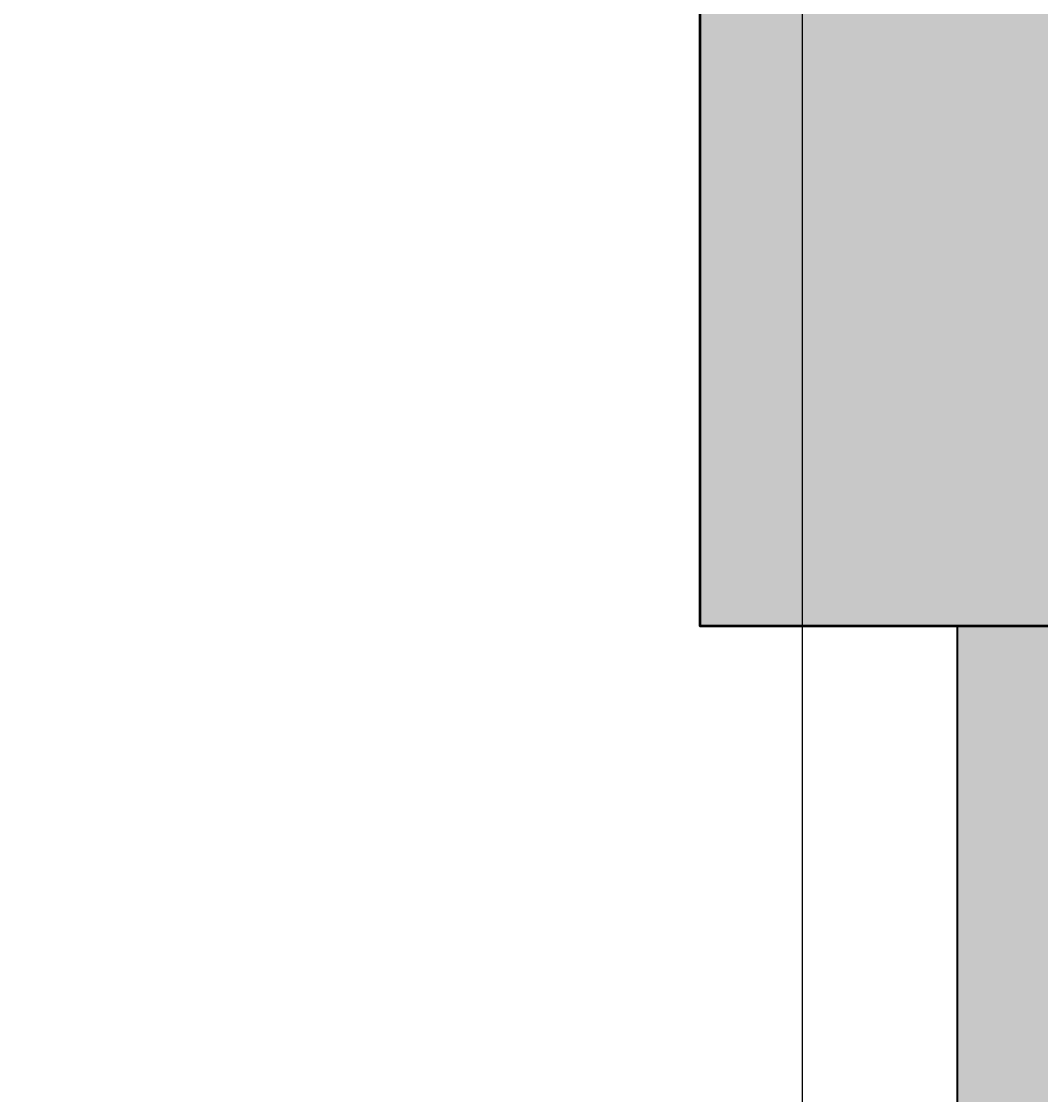
# Model space of a CAD drawing. Units: inches. Extents: x 1998 to 2588, y 1139 to 1977.
# Tile 28 of 134: x 2316 to 2344, y 1456 to 1484. Entities that reach past the tile are written whole.
import ezdxf

# ---------------------------------------------------------------- set-up
doc = ezdxf.new("R2010")
doc.units = ezdxf.units.IN
for name, color, linetype, lineweight in [('A-ANNO-DIMS', 2, 'Continuous', 18), ('A-COLS-PATT', 250, 'Continuous', 13), ('A-WALL-PATT', 252, 'Continuous', 13), ('COLUMN', 10, 'Continuous', 50), ('WALL', 200, 'Continuous', 35)]:
    doc.layers.add(name, color=color, linetype=linetype, lineweight=lineweight)
doc.styles.get("Standard").update_dxf_attribs({"font": 'arial.ttf'})
doc.dimstyles.get("Standard").update_dxf_attribs({"dimtxt": 0.18, "dimasz": 0.18, "dimexe": 0.18, "dimexo": 0.0625, "dimgap": 0.09, "dimtad": 0, "dimtih": 1, "dimtoh": 1, "dimdec": 4, "dimzin": 0, "dimdsep": 46, "dimtxsty": 'Standard', "dimcen": 0.09, "dimadec": 0, "dimazin": 0, "dimtfac": 1, "dimtdec": 4, "dimtofl": 0, "dimtmove": 0, "dimatfit": 3, "dimfxl": 1, "dimtolj": 1, "dimtzin": 0, "dimarcsym": 0})

# ---------------------------------------------------------------- blocks, each defined once
blk = doc.blocks.new('*D23')
at = {"layer": 'A-ANNO-DIMS', "color": 0, "lineweight": -2, "transparency": 16777216}
for p, q in [((2549.179, 1476.17), (2549.179, 1138.602)), ((2059.473, 1413.17), (2059.473, 1138.602)), ((2059.653, 1138.782), (2303.928, 1138.782)), ((2548.999, 1138.782), (2304.723, 1138.782))]:
    blk.add_line(p, q, dxfattribs=at)
at = {"layer": 'A-ANNO-DIMS', "color": 0, "transparency": 16777216}
for points in [[(2059.653, 1138.812), (2059.653, 1138.752), (2059.473, 1138.782)], [(2548.999, 1138.812), (2548.999, 1138.752), (2549.179, 1138.782)]]:
    blk.add_solid(points, dxfattribs=at)
at = {"layer": 'Defpoints', "color": 0, "transparency": 16777216}
for p in [(2549.179, 1476.232), (2059.473, 1413.232), (2549.179, 1138.782)]:
    blk.add_point(p, dxfattribs=at)
at = {"layer": 'A-ANNO-DIMS', "color": 0, "transparency": 16777216, "insert": (2304.326, 1138.782), "char_height": 0.18, "attachment_point": 5}
blk.add_mtext('\\A1;489.7', dxfattribs=at)
blk = doc.blocks.new('*D44')
at = {"layer": 'A-ANNO-DIMS', "color": 0, "lineweight": -2, "transparency": 16777216}
for p, q in [((2295.414, 1588.67), (2295.414, 1138.602)), ((2337.287, 1588.67), (2337.287, 1138.602)), ((2295.594, 1138.782), (2315.953, 1138.782)), ((2337.107, 1138.782), (2316.748, 1138.782))]:
    blk.add_line(p, q, dxfattribs=at)
at = {"layer": 'A-ANNO-DIMS', "color": 0, "transparency": 16777216}
for points in [[(2295.594, 1138.812), (2295.594, 1138.752), (2295.414, 1138.782)], [(2337.107, 1138.812), (2337.107, 1138.752), (2337.287, 1138.782)]]:
    blk.add_solid(points, dxfattribs=at)
at = {"layer": 'Defpoints', "color": 0, "transparency": 16777216}
for p in [(2295.414, 1588.732), (2337.287, 1588.732), (2337.287, 1138.782)]:
    blk.add_point(p, dxfattribs=at)
at = {"layer": 'A-ANNO-DIMS', "color": 0, "transparency": 16777216, "insert": (2316.35, 1138.782), "char_height": 0.18, "attachment_point": 5}
blk.add_mtext('\\A1;41.87', dxfattribs=at)

msp = doc.modelspace()

# ---------------------------------------------------------------- hatches: boundary and pattern name
at = {"layer": 'A-COLS-PATT'}
h = msp.add_hatch(color=256, dxfattribs=at)
h.dxf.hatch_style = 1
h.paths.add_polyline_path([(2099.4125, 1888.7324), (2087.9729, 1888.7324), (2087.9729, 1868.3278), (2099.4125, 1868.3278)])
h.paths.add_polyline_path([(2234.4125, 1888.7324), (2222.9729, 1888.7324), (2222.9729, 1868.3278), (2234.4125, 1868.3278)])
h.paths.add_polyline_path([(2341.4729, 1886.637), (2330.0332, 1886.637), (2330.0332, 1866.2324), (2341.4729, 1866.2324)])
h.paths.add_polyline_path([(2507.8006, 1882.7324), (2487.396, 1882.7324), (2487.396, 1871.2927), (2507.8006, 1871.2927)])
h.paths.add_polyline_path([(2510.9729, 1766.672), (2490.5682, 1766.672), (2490.5682, 1755.2324), (2510.9729, 1755.2324)])
h.paths.add_polyline_path([(2345.9729, 1759.7324), (2334.5332, 1759.7324), (2334.5332, 1739.3278), (2345.9729, 1739.3278)])
h.paths.add_polyline_path([(2234.4125, 1774.3318), (2222.9729, 1774.3318), (2222.9729, 1753.9272), (2234.4125, 1753.9272)])
h.paths.add_polyline_path([(2099.4125, 1775.637), (2087.9729, 1775.637), (2087.9729, 1755.2324), (2099.4125, 1755.2324)])
h.paths.add_polyline_path([(2098.0956, 1593.7241), (2077.691, 1593.7241), (2077.691, 1582.2845), (2098.0956, 1582.2845)])
h.paths.add_polyline_path([(2227.4729, 1604.637), (2216.0332, 1604.637), (2216.0332, 1584.2324), (2227.4729, 1584.2324)])
h.paths.add_polyline_path([(2345.9729, 1647.5211), (2334.5332, 1647.5211), (2334.5332, 1627.1165), (2345.9729, 1627.1165)])
h.paths.add_polyline_path([(2522.3775, 1641.2324), (2501.9729, 1641.2324), (2501.9729, 1629.7927), (2522.3775, 1629.7927)])
h.paths.add_polyline_path([(2522.3775, 1480.7324), (2501.9729, 1480.7324), (2501.9729, 1469.2927), (2522.3775, 1469.2927)])
h.paths.add_polyline_path([(2345.9729, 1488.5616), (2334.5332, 1488.5616), (2334.5332, 1468.1569), (2345.9729, 1468.1569)])
h.paths.add_polyline_path([(2234.4125, 1486.137), (2227.4729, 1486.137), (2227.4729, 1465.7324), (2234.4125, 1465.7324)])
h.paths.add_polyline_path([(2227.4729, 1486.137), (2222.9729, 1486.137), (2222.9729, 1465.7324), (2227.4729, 1465.7324)])
h.paths.add_polyline_path([(2108.3775, 1470.2324), (2087.9729, 1470.2324), (2087.9729, 1458.7927), (2108.3775, 1458.7927)])
h.paths.add_polyline_path([(2096.9729, 1365.5012), (2087.9729, 1365.5012), (2087.9729, 1345.0966), (2096.9729, 1345.0966)])
h.paths.add_polyline_path([(2087.9729, 1365.5012), (2085.5332, 1365.5012), (2085.5332, 1345.0966), (2087.9729, 1345.0966)])
h.paths.add_polyline_path([(2234.4125, 1285.137), (2222.9729, 1285.137), (2222.9729, 1264.7324), (2234.4125, 1264.7324)])
h.paths.add_polyline_path([(2345.9729, 1285.137), (2334.5332, 1285.137), (2334.5332, 1264.7324), (2345.9729, 1264.7324)])
h.paths.add_polyline_path([(2503.1458, 1240.172), (2482.7412, 1240.172), (2482.7412, 1228.7324), (2503.1458, 1228.7324)])
h.paths.add_polyline_path([(2510.9729, 1369.172), (2490.5682, 1369.172), (2490.5682, 1357.7324), (2510.9729, 1357.7324)])
at = {"layer": 'A-WALL-PATT'}
h = msp.add_hatch(color=256, dxfattribs=at)
h.dxf.hatch_style = 1
h.paths.add_polyline_path([(2222.9729, 1888.7324), (2099.4125, 1888.7324), (2099.4125, 1879.7324), (2222.9729, 1879.7324)])
h.paths.add_polyline_path([(2096.9729, 1868.3278), (2087.9729, 1868.3278), (2087.9729, 1775.637), (2096.9729, 1775.637)])
h.paths.add_polyline_path([(2227.4729, 1868.3278), (2222.9729, 1868.3278), (2222.9729, 1774.3318), (2227.4729, 1774.3318)])
h.paths.add_polyline_path([(2188.3019, 1759.7324), (2138.6074, 1759.7324), (2099.4125, 1759.7324), (2099.4125, 1755.2324), (2176.9729, 1755.2324), (2188.3019, 1755.2324)])
h.paths.add_polyline_path([(2087.9729, 1759.7324), (2059.4729, 1759.7324), (2059.4729, 1702.7324), (2087.9729, 1702.7324), (2087.9729, 1707.2324), (2063.9729, 1707.2324), (2063.9729, 1755.2324), (2087.9729, 1755.2324)])
h.paths.add_polyline_path([(2096.9729, 1755.2324), (2087.9729, 1755.2324), (2087.9729, 1707.2324), (2096.9729, 1707.2324)])
h.paths.add_polyline_path([(2187.0461, 1707.2324), (2105.9729, 1707.2324), (2096.9729, 1707.2324), (2087.9729, 1707.2324), (2087.9729, 1702.7324), (2105.9729, 1702.7324), (2114.9729, 1702.7324), (2187.0461, 1702.7324)])
h.paths.add_polyline_path([(2181.4729, 1719.2028), (2176.9729, 1719.2028), (2176.9729, 1707.2324), (2181.4729, 1707.2324)])
h.paths.add_polyline_path([(2216.0332, 1588.7324), (2114.9729, 1588.7324), (2105.9729, 1588.7324), (2105.9729, 1584.2324), (2216.0332, 1584.2324)])
h.paths.add_polyline_path([(2077.691, 1588.7324), (2061.4729, 1588.7324), (2061.4729, 1584.2324), (2077.691, 1584.2324)])
h.paths.add_polyline_path([(2105.9729, 1588.7324), (2098.0956, 1588.7324), (2098.0956, 1584.2324), (2105.9729, 1584.2324)])
h.paths.add_polyline_path([(2114.9729, 1596.2642), (2110.1012, 1596.2642), (2105.9729, 1596.2642), (2105.9729, 1588.7324), (2114.9729, 1588.7324)])
h.paths.add_polyline_path([(2114.9729, 1584.2324), (2105.9729, 1584.2324), (2105.9729, 1580.249), (2110.1012, 1580.249), (2114.9729, 1580.249)])
h.paths.add_polyline_path([(2114.9729, 1547.7716), (2110.1012, 1547.7716, -0.0318759), (2105.9729, 1548.035), (2105.9729, 1470.2324), (2108.3775, 1470.2324), (2108.3775, 1465.7324), (2186.2943, 1465.7324), (2186.2943, 1470.2324), (2114.9729, 1470.2324)])
h.paths.add_polyline_path([(2227.4729, 1584.2324), (2222.9729, 1584.2324), (2222.9729, 1486.137), (2227.4729, 1486.137)])
h.paths.add_polyline_path([(2295.4138, 1593.2324), (2227.4729, 1593.2324), (2227.4729, 1588.7324), (2295.4138, 1588.7324), (2295.4138, 1591.8729)])
h.paths.add_polyline_path([(2345.9729, 1627.1165), (2341.4729, 1627.1165), (2341.4729, 1593.2324), (2337.2869, 1593.2324), (2337.2869, 1591.8729), (2337.2869, 1588.7324), (2345.9729, 1588.7324)])
h.paths.add_polyline_path([(2291.9729, 1588.7324), (2287.4729, 1588.7324), (2287.4729, 1522.7324), (2291.9729, 1522.7324)])
h.paths.add_polyline_path([(2291.9729, 1522.7324), (2287.4729, 1522.7324), (2227.4729, 1522.7324), (2227.4729, 1518.2324), (2291.9729, 1518.2324)])
h.paths.add_polyline_path([(2295.7347, 1519.5919), (2295.7347, 1522.7324), (2291.9729, 1522.7324), (2291.9729, 1518.2324), (2295.7347, 1518.2324)])
h.paths.add_polyline_path([(2345.9729, 1522.7324), (2337.6078, 1522.7324), (2337.6078, 1519.5919), (2337.6078, 1518.2324), (2341.4729, 1518.2324), (2341.4729, 1488.5616), (2345.9729, 1488.5616)])
h.paths.add_polyline_path([(2345.9729, 1468.1569), (2341.4729, 1468.1569), (2341.4729, 1374.2324), (2227.4729, 1374.2324), (2227.4729, 1369.7324), (2345.9729, 1369.7324)])
h.paths.add_polyline_path([(2345.9729, 1369.7324), (2341.4729, 1369.7324), (2341.4729, 1362.2324), (2345.9729, 1362.2324)])
h.paths.add_polyline_path([(2345.9729, 1317.7324), (2345.9729, 1322.2324), (2341.4729, 1322.2324), (2341.4729, 1285.137), (2345.9729, 1285.137)], flags=17)
h.paths.add_polyline_path([(2356.2096, 1322.2324), (2345.9729, 1322.2324), (2345.9729, 1317.7324), (2356.2096, 1317.7324), (2356.2096, 1319.3088)], flags=17)
h.paths.add_polyline_path([(2393.9729, 1322.2324), (2375.6999, 1322.2324), (2375.6999, 1319.3088, -0.0202458), (2375.636, 1317.7324), (2393.9729, 1317.7324)], flags=17)
h.paths.add_polyline_path([(2398.4729, 1322.2324), (2393.9729, 1322.2324), (2393.9729, 1317.7324), (2393.9729, 1237.7324), (2345.9729, 1237.7324), (2345.9729, 1264.7324), (2341.4729, 1264.7324), (2341.4729, 1228.7324), (2393.9729, 1228.7324), (2482.7412, 1228.7324), (2482.7412, 1237.7324), (2398.4729, 1237.7324), (2398.4729, 1297.1029)])
h.paths.add_polyline_path([(2398.4729, 1362.2324), (2393.9729, 1362.2324), (2393.9729, 1357.7324), (2398.4729, 1357.7324)])
h.paths.add_polyline_path([(2345.9729, 1329.7549), (2341.4729, 1329.7549), (2341.4729, 1322.2324), (2345.9729, 1322.2324)])

# ---------------------------------------------------------------- linework, layer by layer
at = {"layer": 'COLUMN'}
msp.add_lwpolyline([(2334.5332, 1488.5616), (2345.9729, 1488.5616), (2345.9729, 1468.1569), (2334.5332, 1468.1569)], close=True, dxfattribs=at)
at = {"layer": 'WALL'}
msp.add_line((2341.4729, 1468.1569), (2341.4729, 1374.2324), dxfattribs=at)

# ---------------------------------------------------------------- dimensions: what is measured, and where the dimension line sits
at = {"layer": 'A-ANNO-DIMS'}
for base, p1, p2, override, picture, middle in [((2337.2869, 1138.7824), (2295.4138, 1588.7324), (2337.2869, 1588.7324), {"dimdec": 2, "dimlfac": 1, "dimrnd": 0, "dimzin": 0, "dimdsep": 46, "dimlunit": 2}, '*D44', (2316.3503, 1138.7824)), ((2549.1786, 1138.7824), (2059.4729, 1413.2324), (2549.1786, 1476.2324), {"dimdec": 1, "dimlfac": 1, "dimrnd": 0, "dimzin": 0, "dimdsep": 46, "dimlunit": 2}, '*D23', (2304.3257, 1138.7824))]:
    dim = msp.add_linear_dim(base=base, p1=p1, p2=p2, dimstyle='Standard', override=override, dxfattribs=at)
    dim.commit()
    dim.dimension.update_dxf_attribs({"geometry": picture, "text_midpoint": middle})

doc.saveas('drawing.dxf')
